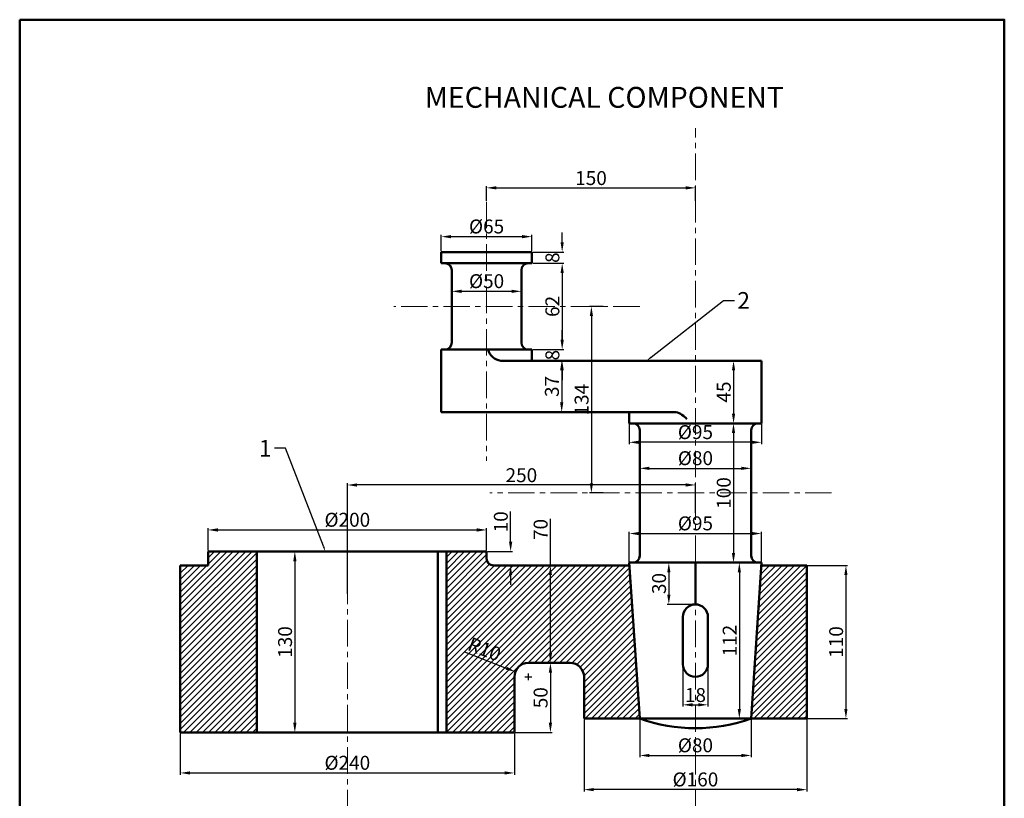
# Model space of a CAD drawing. Units: millimetres. Extents: x 1219 to 1926, y 574 to 1498.
# Tile 2 of 2: x 1219 to 1926, y 938 to 1498. Entities that reach past the tile are written whole.
import ezdxf
from ezdxf import colors
from ezdxf.entities.mleader import LeaderData, LeaderLine
from ezdxf.math import Vec2, Vec3

# ---------------------------------------------------------------- set-up
doc = ezdxf.new("R2010")
doc.units = ezdxf.units.MM
doc.header["$LTSCALE"] = 0.6
doc.linetypes.add('CENTER', pattern=[50.8, 31.75, -6.35, 6.35, -6.35])
for name, color, linetype, lineweight in [('M-CNTR', 1, 'CENTER', 18), ('M-DIMS', 2, 'Continuous', 25), ('M-HATC', 8, 'Continuous', 18), ('M-OUTL', 7, 'Continuous', 50), ('M-TEXT', 3, 'Continuous', 25), ('M-TTLB', 7, 'Continuous', 50)]:
    doc.layers.add(name, color=color, linetype=linetype, lineweight=lineweight)
doc.styles.get("Standard").update_dxf_attribs({"font": 'arial.ttf'})
doc.dimstyles.new('ISO-25', dxfattribs={"dimtxt": 10, "dimasz": 7, "dimexe": 1.25, "dimexo": 0.625, "dimtad": 1, "dimdec": 0, "dimtxsty": 'Standard', "dimcen": 2.5, "dimadec": 0, "dimazin": 0, "dimtfac": 1, "dimtdec": 0, "dimtofl": 0, "dimtmove": 0, "dimatfit": 3, "dimfxl": 1, "dimarcsym": 0})

# ---------------------------------------------------------------- blocks, each defined once
blk = doc.blocks.new('*D1')
at = {"layer": 'Defpoints', "color": 0, "ltscale": 0.6, "transparency": 16777216}
for p in [(1586.44, 1341.72), (1521.44, 1330.65), (1586.44, 1330.65)]:
    blk.add_point(p, dxfattribs=at)
at = {"layer": 'M-DIMS', "color": 0, "lineweight": -2, "ltscale": 0.6, "transparency": 16777216}
for p, q in [((1521.44, 1331.27), (1521.44, 1342.97)), ((1528.44, 1341.72), (1579.44, 1341.72)), ((1586.44, 1331.27), (1586.44, 1342.97))]:
    blk.add_line(p, q, dxfattribs=at)
at = {"layer": 'M-DIMS', "color": 0, "ltscale": 0.6, "transparency": 16777216}
for points in [[(1528.44, 1342.88), (1528.44, 1340.55), (1521.44, 1341.72)], [(1579.44, 1342.88), (1579.44, 1340.55), (1586.44, 1341.72)]]:
    blk.add_solid(points, dxfattribs=at)
at = {"layer": 'M-DIMS', "color": 0, "ltscale": 0.6, "transparency": 16777216, "insert": (1553.94, 1347.73), "char_height": 10, "attachment_point": 5}
blk.add_mtext('%%C65', dxfattribs=at)
blk = doc.blocks.new('*D2')
at = {"layer": 'Defpoints', "color": 0, "ltscale": 0.6, "transparency": 16777216}
for p in [(1703.94, 1376.76), (1553.94, 1366.8), (1703.94, 1366.8)]:
    blk.add_point(p, dxfattribs=at)
at = {"layer": 'M-DIMS', "color": 0, "lineweight": -2, "ltscale": 0.6, "transparency": 16777216}
for p, q in [((1553.94, 1367.43), (1553.94, 1378.01)), ((1560.94, 1376.76), (1696.94, 1376.76)), ((1703.94, 1367.43), (1703.94, 1378.01))]:
    blk.add_line(p, q, dxfattribs=at)
at = {"layer": 'M-DIMS', "color": 0, "ltscale": 0.6, "transparency": 16777216}
for points in [[(1560.94, 1377.93), (1560.94, 1375.6), (1553.94, 1376.76)], [(1696.94, 1377.93), (1696.94, 1375.6), (1703.94, 1376.76)]]:
    blk.add_solid(points, dxfattribs=at)
at = {"layer": 'M-DIMS', "color": 0, "ltscale": 0.6, "transparency": 16777216, "insert": (1628.94, 1382.49), "char_height": 10, "attachment_point": 5}
blk.add_mtext('150', dxfattribs=at)
blk = doc.blocks.new('*D3')
at = {"layer": 'Defpoints', "color": 0, "ltscale": 0.6, "transparency": 16777216}
for p in [(1586.44, 1330.65), (1586.44, 1322.65), (1608.23, 1322.65)]:
    blk.add_point(p, dxfattribs=at)
at = {"layer": 'M-DIMS', "color": 0, "lineweight": -2, "ltscale": 0.6, "transparency": 16777216}
for p, q in [((1608.23, 1337.65), (1608.23, 1344.65)), ((1587.07, 1330.65), (1609.48, 1330.65)), ((1587.07, 1322.65), (1609.48, 1322.65)), ((1608.23, 1315.65), (1608.23, 1308.65))]:
    blk.add_line(p, q, dxfattribs=at)
at = {"layer": 'M-DIMS', "color": 0, "ltscale": 0.6, "transparency": 16777216}
for points in [[(1607.06, 1337.65), (1609.4, 1337.65), (1608.23, 1330.65)], [(1607.06, 1315.65), (1609.4, 1315.65), (1608.23, 1322.65)]]:
    blk.add_solid(points, dxfattribs=at)
at = {"layer": 'M-DIMS', "color": 0, "ltscale": 0.6, "transparency": 16777216, "insert": (1602.5, 1326.65), "char_height": 10, "attachment_point": 5, "rotation": 90}
blk.add_mtext('8', dxfattribs=at)
blk = doc.blocks.new('*D4')
at = {"layer": 'Defpoints', "color": 0, "ltscale": 0.6, "transparency": 16777216}
for p in [(1586.44, 1322.65), (1586.44, 1260.65), (1608.23, 1260.65)]:
    blk.add_point(p, dxfattribs=at)
at = {"layer": 'M-DIMS', "color": 0, "lineweight": -2, "ltscale": 0.6, "transparency": 16777216}
for p, q in [((1587.07, 1322.65), (1609.48, 1322.65)), ((1608.23, 1315.65), (1608.23, 1267.65)), ((1587.07, 1260.65), (1609.48, 1260.65))]:
    blk.add_line(p, q, dxfattribs=at)
at = {"layer": 'M-DIMS', "color": 0, "ltscale": 0.6, "transparency": 16777216}
for points in [[(1607.06, 1315.65), (1609.4, 1315.65), (1608.23, 1322.65)], [(1607.06, 1267.65), (1609.4, 1267.65), (1608.23, 1260.65)]]:
    blk.add_solid(points, dxfattribs=at)
at = {"layer": 'M-DIMS', "color": 0, "ltscale": 0.6, "transparency": 16777216, "insert": (1602.5, 1291.65), "char_height": 10, "attachment_point": 5, "rotation": 90}
blk.add_mtext('62', dxfattribs=at)
blk = doc.blocks.new('*D5')
at = {"layer": 'Defpoints', "color": 0, "ltscale": 0.6, "transparency": 16777216}
for p in [(1586.44, 1260.65), (1586.44, 1252.65), (1608.23, 1252.65)]:
    blk.add_point(p, dxfattribs=at)
at = {"layer": 'M-DIMS', "color": 0, "lineweight": -2, "ltscale": 0.6, "transparency": 16777216}
for p, q in [((1608.23, 1267.65), (1608.23, 1274.65)), ((1587.07, 1260.65), (1609.48, 1260.65)), ((1587.07, 1252.65), (1609.48, 1252.65)), ((1608.23, 1245.65), (1608.23, 1238.65))]:
    blk.add_line(p, q, dxfattribs=at)
at = {"layer": 'M-DIMS', "color": 0, "ltscale": 0.6, "transparency": 16777216}
for points in [[(1607.06, 1267.65), (1609.4, 1267.65), (1608.23, 1260.65)], [(1607.06, 1245.65), (1609.4, 1245.65), (1608.23, 1252.65)]]:
    blk.add_solid(points, dxfattribs=at)
at = {"layer": 'M-DIMS', "color": 0, "ltscale": 0.6, "transparency": 16777216, "insert": (1602.5, 1256.65), "char_height": 10, "attachment_point": 5, "rotation": 90}
blk.add_mtext('8', dxfattribs=at)
blk = doc.blocks.new('*D6')
at = {"layer": 'Defpoints', "color": 0, "ltscale": 0.6, "transparency": 16777216}
for p in [(1616.05, 1252.65), (1607.9, 1215.65), (1616.05, 1215.65)]:
    blk.add_point(p, dxfattribs=at)
at = {"layer": 'M-DIMS', "color": 0, "lineweight": -2, "ltscale": 0.6, "transparency": 16777216}
for p, q in [((1615.42, 1252.65), (1606.65, 1252.65)), ((1607.9, 1245.65), (1607.9, 1222.65)), ((1615.42, 1215.65), (1606.65, 1215.65))]:
    blk.add_line(p, q, dxfattribs=at)
at = {"layer": 'M-DIMS', "color": 0, "ltscale": 0.6, "transparency": 16777216}
for points in [[(1606.73, 1245.65), (1609.06, 1245.65), (1607.9, 1252.65)], [(1606.73, 1222.65), (1609.06, 1222.65), (1607.9, 1215.65)]]:
    blk.add_solid(points, dxfattribs=at)
at = {"layer": 'M-DIMS', "color": 0, "ltscale": 0.6, "transparency": 16777216, "insert": (1602.16, 1234.15), "char_height": 10, "attachment_point": 5, "rotation": 90}
blk.add_mtext('37', dxfattribs=at)
blk = doc.blocks.new('*D7')
at = {"layer": 'Defpoints', "color": 0, "ltscale": 0.6, "transparency": 16777216}
for p in [(1638.23, 1291.65), (1629.22, 1157.65), (1638.23, 1157.65)]:
    blk.add_point(p, dxfattribs=at)
at = {"layer": 'M-DIMS', "color": 0, "lineweight": -2, "ltscale": 0.6, "transparency": 16777216}
for p, q in [((1637.61, 1291.65), (1627.97, 1291.65)), ((1629.22, 1284.65), (1629.22, 1164.65)), ((1637.61, 1157.65), (1627.97, 1157.65))]:
    blk.add_line(p, q, dxfattribs=at)
at = {"layer": 'M-DIMS', "color": 0, "ltscale": 0.6, "transparency": 16777216}
for points in [[(1628.06, 1284.65), (1630.39, 1284.65), (1629.22, 1291.65)], [(1628.06, 1164.65), (1630.39, 1164.65), (1629.22, 1157.65)]]:
    blk.add_solid(points, dxfattribs=at)
at = {"layer": 'M-DIMS', "color": 0, "ltscale": 0.6, "transparency": 16777216, "insert": (1623.49, 1224.65), "char_height": 10, "attachment_point": 5, "rotation": 90}
blk.add_mtext('134', dxfattribs=at)
blk = doc.blocks.new('*D8')
at = {"layer": 'Defpoints', "color": 0, "ltscale": 0.6, "transparency": 16777216}
for p in [(1528.94, 1303.11), (1578.94, 1303.11), (1578.94, 1302.46)]:
    blk.add_point(p, dxfattribs=at)
at = {"layer": 'M-DIMS', "color": 0, "lineweight": -2, "ltscale": 0.6, "transparency": 16777216}
for p, q in [((1528.94, 1302.48), (1528.94, 1301.21)), ((1535.94, 1302.46), (1571.94, 1302.46)), ((1578.94, 1302.48), (1578.94, 1301.21))]:
    blk.add_line(p, q, dxfattribs=at)
at = {"layer": 'M-DIMS', "color": 0, "ltscale": 0.6, "transparency": 16777216}
for points in [[(1535.94, 1303.63), (1535.94, 1301.29), (1528.94, 1302.46)], [(1571.94, 1303.63), (1571.94, 1301.29), (1578.94, 1302.46)]]:
    blk.add_solid(points, dxfattribs=at)
at = {"layer": 'M-DIMS', "color": 0, "ltscale": 0.6, "transparency": 16777216, "insert": (1553.94, 1308.47), "char_height": 10, "attachment_point": 5}
blk.add_mtext('%%C50', dxfattribs=at)
blk = doc.blocks.new('*D9')
at = {"layer": 'Defpoints', "color": 0, "ltscale": 0.6, "transparency": 16777216}
for p in [(1728.88, 1252.65), (1728.88, 1207.65), (1731.3, 1207.65)]:
    blk.add_point(p, dxfattribs=at)
at = {"layer": 'M-DIMS', "color": 0, "lineweight": -2, "ltscale": 0.6, "transparency": 16777216}
for p, q in [((1729.5, 1252.65), (1732.55, 1252.65)), ((1731.3, 1245.65), (1731.3, 1214.65)), ((1729.5, 1207.65), (1732.55, 1207.65))]:
    blk.add_line(p, q, dxfattribs=at)
at = {"layer": 'M-DIMS', "color": 0, "ltscale": 0.6, "transparency": 16777216}
for points in [[(1730.14, 1245.65), (1732.47, 1245.65), (1731.3, 1252.65)], [(1730.14, 1214.65), (1732.47, 1214.65), (1731.3, 1207.65)]]:
    blk.add_solid(points, dxfattribs=at)
at = {"layer": 'M-DIMS', "color": 0, "ltscale": 0.6, "transparency": 16777216, "insert": (1725.59, 1230.15), "char_height": 10, "attachment_point": 5, "rotation": 90}
blk.add_mtext('45', dxfattribs=at)
blk = doc.blocks.new('*D10')
at = {"layer": 'Defpoints', "color": 0, "ltscale": 0.6, "transparency": 16777216}
for p in [(1656.44, 1207.65), (1751.44, 1207.65), (1656.44, 1194.05)]:
    blk.add_point(p, dxfattribs=at)
at = {"layer": 'M-DIMS', "color": 0, "lineweight": -2, "ltscale": 0.6, "transparency": 16777216}
for p, q in [((1656.44, 1207.02), (1656.44, 1192.8)), ((1751.44, 1207.02), (1751.44, 1192.8)), ((1744.44, 1194.05), (1663.44, 1194.05))]:
    blk.add_line(p, q, dxfattribs=at)
at = {"layer": 'M-DIMS', "color": 0, "ltscale": 0.6, "transparency": 16777216}
for points in [[(1663.44, 1195.22), (1663.44, 1192.88), (1656.44, 1194.05)], [(1744.44, 1195.22), (1744.44, 1192.88), (1751.44, 1194.05)]]:
    blk.add_solid(points, dxfattribs=at)
at = {"layer": 'M-DIMS', "color": 0, "ltscale": 0.6, "transparency": 16777216, "insert": (1703.94, 1200.06), "char_height": 10, "attachment_point": 5}
blk.add_mtext('%%C95', dxfattribs=at)
blk = doc.blocks.new('*D11')
at = {"layer": 'Defpoints', "color": 0, "ltscale": 0.6, "transparency": 16777216}
for p in [(1663.94, 1175.97), (1743.94, 1175.97), (1743.94, 1175.35)]:
    blk.add_point(p, dxfattribs=at)
at = {"layer": 'M-DIMS', "color": 0, "lineweight": -2, "ltscale": 0.6, "transparency": 16777216}
for p, q in [((1663.94, 1175.35), (1663.94, 1174.1)), ((1670.94, 1175.35), (1736.94, 1175.35)), ((1743.94, 1175.35), (1743.94, 1174.1))]:
    blk.add_line(p, q, dxfattribs=at)
at = {"layer": 'M-DIMS', "color": 0, "ltscale": 0.6, "transparency": 16777216}
for points in [[(1670.94, 1176.52), (1670.94, 1174.19), (1663.94, 1175.35)], [(1736.94, 1176.52), (1736.94, 1174.19), (1743.94, 1175.35)]]:
    blk.add_solid(points, dxfattribs=at)
at = {"layer": 'M-DIMS', "color": 0, "ltscale": 0.6, "transparency": 16777216, "insert": (1703.94, 1181.36), "char_height": 10, "attachment_point": 5}
blk.add_mtext('%%C80', dxfattribs=at)
blk = doc.blocks.new('*D12')
at = {"layer": 'Defpoints', "color": 0, "ltscale": 0.6, "transparency": 16777216}
for p in [(1731.03, 1207.65), (1731.03, 1107.65), (1731.29, 1107.65)]:
    blk.add_point(p, dxfattribs=at)
at = {"layer": 'M-DIMS', "color": 0, "lineweight": -2, "ltscale": 0.6, "transparency": 16777216}
for p, q in [((1731.65, 1207.65), (1732.54, 1207.65)), ((1731.29, 1200.65), (1731.29, 1114.65)), ((1731.65, 1107.65), (1732.54, 1107.65))]:
    blk.add_line(p, q, dxfattribs=at)
at = {"layer": 'M-DIMS', "color": 0, "ltscale": 0.6, "transparency": 16777216}
for points in [[(1730.12, 1200.65), (1732.46, 1200.65), (1731.29, 1207.65)], [(1730.12, 1114.65), (1732.46, 1114.65), (1731.29, 1107.65)]]:
    blk.add_solid(points, dxfattribs=at)
at = {"layer": 'M-DIMS', "color": 0, "ltscale": 0.6, "transparency": 16777216, "insert": (1725.56, 1157.65), "char_height": 10, "attachment_point": 5, "rotation": 90}
blk.add_mtext('100', dxfattribs=at)
blk = doc.blocks.new('*D13')
at = {"layer": 'Defpoints', "color": 0, "ltscale": 0.6, "transparency": 16777216}
for p in [(1751.44, 1128.54), (1656.44, 1107.65), (1751.44, 1107.65)]:
    blk.add_point(p, dxfattribs=at)
at = {"layer": 'M-DIMS', "color": 0, "lineweight": -2, "ltscale": 0.6, "transparency": 16777216}
for p, q in [((1656.44, 1108.27), (1656.44, 1129.79)), ((1663.44, 1128.54), (1744.44, 1128.54)), ((1751.44, 1108.27), (1751.44, 1129.79))]:
    blk.add_line(p, q, dxfattribs=at)
at = {"layer": 'M-DIMS', "color": 0, "ltscale": 0.6, "transparency": 16777216}
for points in [[(1663.44, 1129.7), (1663.44, 1127.37), (1656.44, 1128.54)], [(1744.44, 1129.7), (1744.44, 1127.37), (1751.44, 1128.54)]]:
    blk.add_solid(points, dxfattribs=at)
at = {"layer": 'M-DIMS', "color": 0, "ltscale": 0.6, "transparency": 16777216, "insert": (1703.94, 1134.55), "char_height": 10, "attachment_point": 5}
blk.add_mtext('%%C95', dxfattribs=at)
blk = doc.blocks.new('*D14')
at = {"layer": 'Defpoints', "color": 0, "ltscale": 0.6, "transparency": 16777216}
for p in [(1703.94, 1107.65), (1684.83, 1077.65), (1703.94, 1077.65)]:
    blk.add_point(p, dxfattribs=at)
at = {"layer": 'M-DIMS', "color": 0, "lineweight": -2, "ltscale": 0.6, "transparency": 16777216}
for p, q in [((1703.32, 1107.65), (1683.58, 1107.65)), ((1684.83, 1100.65), (1684.83, 1084.65)), ((1703.32, 1077.65), (1683.58, 1077.65))]:
    blk.add_line(p, q, dxfattribs=at)
at = {"layer": 'M-DIMS', "color": 0, "ltscale": 0.6, "transparency": 16777216}
for points in [[(1683.67, 1100.65), (1686, 1100.65), (1684.83, 1107.65)], [(1683.67, 1084.65), (1686, 1084.65), (1684.83, 1077.65)]]:
    blk.add_solid(points, dxfattribs=at)
at = {"layer": 'M-DIMS', "color": 0, "ltscale": 0.6, "transparency": 16777216, "insert": (1679.1, 1092.65), "char_height": 10, "attachment_point": 5, "rotation": 90}
blk.add_mtext('30', dxfattribs=at)
blk = doc.blocks.new('*D15')
at = {"layer": 'Defpoints', "color": 0, "ltscale": 0.6, "transparency": 16777216}
for p in [(1731.03, 1107.65), (1731.03, 995.65), (1735.48, 995.65)]:
    blk.add_point(p, dxfattribs=at)
at = {"layer": 'M-DIMS', "color": 0, "lineweight": -2, "ltscale": 0.6, "transparency": 16777216}
for p, q in [((1731.65, 1107.65), (1736.73, 1107.65)), ((1735.48, 1100.65), (1735.48, 1002.65)), ((1731.65, 995.65), (1736.73, 995.65))]:
    blk.add_line(p, q, dxfattribs=at)
at = {"layer": 'M-DIMS', "color": 0, "ltscale": 0.6, "transparency": 16777216}
for points in [[(1734.31, 1100.65), (1736.65, 1100.65), (1735.48, 1107.65)], [(1734.31, 1002.65), (1736.65, 1002.65), (1735.48, 995.65)]]:
    blk.add_solid(points, dxfattribs=at)
at = {"layer": 'M-DIMS', "color": 0, "ltscale": 0.6, "transparency": 16777216, "insert": (1729.83, 1051.65), "char_height": 10, "attachment_point": 5, "rotation": 90}
blk.add_mtext('112', dxfattribs=at)
blk = doc.blocks.new('*D16')
at = {"layer": 'Defpoints', "color": 0, "ltscale": 0.6, "transparency": 16777216}
for p in [(1694.94, 1043.46), (1712.94, 1043.46), (1712.94, 1005.56)]:
    blk.add_point(p, dxfattribs=at)
at = {"layer": 'M-DIMS', "color": 0, "lineweight": -2, "ltscale": 0.6, "transparency": 16777216}
for p, q in [((1694.94, 1042.83), (1694.94, 1004.31)), ((1712.94, 1042.83), (1712.94, 1004.31)), ((1701.94, 1005.56), (1705.94, 1005.56))]:
    blk.add_line(p, q, dxfattribs=at)
at = {"layer": 'M-DIMS', "color": 0, "ltscale": 0.6, "transparency": 16777216}
for points in [[(1701.94, 1006.72), (1701.94, 1004.39), (1694.94, 1005.56)], [(1705.94, 1006.72), (1705.94, 1004.39), (1712.94, 1005.56)]]:
    blk.add_solid(points, dxfattribs=at)
at = {"layer": 'M-DIMS', "color": 0, "ltscale": 0.6, "transparency": 16777216, "insert": (1703.94, 1011.29), "char_height": 10, "attachment_point": 5}
blk.add_mtext('18', dxfattribs=at)
blk = doc.blocks.new('*D17')
at = {"layer": 'Defpoints', "color": 0, "ltscale": 0.6, "transparency": 16777216}
for p in [(1767.63, 1105.65), (1767.63, 995.65), (1812.01, 995.65)]:
    blk.add_point(p, dxfattribs=at)
at = {"layer": 'M-DIMS', "color": 0, "lineweight": -2, "ltscale": 0.6, "transparency": 16777216}
for p, q in [((1768.25, 1105.65), (1813.26, 1105.65)), ((1812.01, 1098.65), (1812.01, 1002.65)), ((1768.25, 995.65), (1813.26, 995.65))]:
    blk.add_line(p, q, dxfattribs=at)
at = {"layer": 'M-DIMS', "color": 0, "ltscale": 0.6, "transparency": 16777216}
for points in [[(1810.84, 1098.65), (1813.18, 1098.65), (1812.01, 1105.65)], [(1810.84, 1002.65), (1813.18, 1002.65), (1812.01, 995.65)]]:
    blk.add_solid(points, dxfattribs=at)
at = {"layer": 'M-DIMS', "color": 0, "ltscale": 0.6, "transparency": 16777216, "insert": (1806.28, 1050.65), "char_height": 10, "attachment_point": 5, "rotation": 90}
blk.add_mtext('110', dxfattribs=at)
blk = doc.blocks.new('*D18')
at = {"layer": 'Defpoints', "color": 0, "ltscale": 0.6, "transparency": 16777216}
for p in [(1553.94, 1131.12), (1353.94, 1115.65), (1553.94, 1115.65)]:
    blk.add_point(p, dxfattribs=at)
at = {"layer": 'M-DIMS', "color": 0, "lineweight": -2, "ltscale": 0.6, "transparency": 16777216}
for p, q in [((1353.94, 1116.27), (1353.94, 1132.37)), ((1553.94, 1116.27), (1553.94, 1132.37)), ((1360.94, 1131.12), (1546.94, 1131.12))]:
    blk.add_line(p, q, dxfattribs=at)
at = {"layer": 'M-DIMS', "color": 0, "ltscale": 0.6, "transparency": 16777216}
for points in [[(1360.94, 1132.29), (1360.94, 1129.95), (1353.94, 1131.12)], [(1546.94, 1132.29), (1546.94, 1129.95), (1553.94, 1131.12)]]:
    blk.add_solid(points, dxfattribs=at)
at = {"layer": 'M-DIMS', "color": 0, "ltscale": 0.6, "transparency": 16777216, "insert": (1453.94, 1137.13), "char_height": 10, "attachment_point": 5}
blk.add_mtext('%%C200', dxfattribs=at)
blk = doc.blocks.new('*D19')
at = {"layer": 'Defpoints', "color": 0, "ltscale": 0.6, "transparency": 16777216}
for p in [(1453.94, 1163.41), (1703.94, 1142.52), (1453.94, 1084.55)]:
    blk.add_point(p, dxfattribs=at)
at = {"layer": 'M-DIMS', "color": 0, "lineweight": -2, "ltscale": 0.6, "transparency": 16777216}
for p, q in [((1453.94, 1085.17), (1453.94, 1164.66)), ((1696.94, 1163.41), (1460.94, 1163.41)), ((1703.94, 1143.14), (1703.94, 1164.66))]:
    blk.add_line(p, q, dxfattribs=at)
at = {"layer": 'M-DIMS', "color": 0, "ltscale": 0.6, "transparency": 16777216}
for points in [[(1460.94, 1164.57), (1460.94, 1162.24), (1453.94, 1163.41)], [(1696.94, 1164.57), (1696.94, 1162.24), (1703.94, 1163.41)]]:
    blk.add_solid(points, dxfattribs=at)
at = {"layer": 'M-DIMS', "color": 0, "ltscale": 0.6, "transparency": 16777216, "insert": (1578.94, 1169.14), "char_height": 10, "attachment_point": 5}
blk.add_mtext('250', dxfattribs=at)
blk = doc.blocks.new('*D20')
at = {"layer": 'Defpoints', "color": 0, "ltscale": 0.6, "transparency": 16777216}
for p in [(1333.94, 985.65), (1573.94, 985.65), (1573.94, 956.62)]:
    blk.add_point(p, dxfattribs=at)
at = {"layer": 'M-DIMS', "color": 0, "lineweight": -2, "ltscale": 0.6, "transparency": 16777216}
for p, q in [((1333.94, 985.02), (1333.94, 955.37)), ((1573.94, 985.02), (1573.94, 955.37)), ((1340.94, 956.62), (1566.94, 956.62))]:
    blk.add_line(p, q, dxfattribs=at)
at = {"layer": 'M-DIMS', "color": 0, "ltscale": 0.6, "transparency": 16777216}
for points in [[(1340.94, 957.79), (1340.94, 955.46), (1333.94, 956.62)], [(1566.94, 957.79), (1566.94, 955.46), (1573.94, 956.62)]]:
    blk.add_solid(points, dxfattribs=at)
at = {"layer": 'M-DIMS', "color": 0, "ltscale": 0.6, "transparency": 16777216, "insert": (1453.94, 962.63), "char_height": 10, "attachment_point": 5}
blk.add_mtext('%%C240', dxfattribs=at)
blk = doc.blocks.new('*D21')
at = {"layer": 'Defpoints', "color": 0, "ltscale": 0.6, "transparency": 16777216}
for p in [(1416.57, 1115.65), (1416.23, 985.65), (1416.57, 985.65)]:
    blk.add_point(p, dxfattribs=at)
at = {"layer": 'M-DIMS', "color": 0, "lineweight": -2, "ltscale": 0.6, "transparency": 16777216}
for p, q in [((1415.94, 1115.65), (1414.98, 1115.65)), ((1416.23, 1108.65), (1416.23, 992.65)), ((1415.94, 985.65), (1414.98, 985.65))]:
    blk.add_line(p, q, dxfattribs=at)
at = {"layer": 'M-DIMS', "color": 0, "ltscale": 0.6, "transparency": 16777216}
for points in [[(1415.07, 1108.65), (1417.4, 1108.65), (1416.23, 1115.65)], [(1415.07, 992.65), (1417.4, 992.65), (1416.23, 985.65)]]:
    blk.add_solid(points, dxfattribs=at)
at = {"layer": 'M-DIMS', "color": 0, "ltscale": 0.6, "transparency": 16777216, "insert": (1410.5, 1050.65), "char_height": 10, "attachment_point": 5, "rotation": 90}
blk.add_mtext('130', dxfattribs=at)
blk = doc.blocks.new('*D22')
at = {"layer": 'Defpoints', "color": 0, "ltscale": 0.6, "transparency": 16777216}
for p in [(1623.94, 995.65), (1783.94, 995.65), (1623.94, 944.65)]:
    blk.add_point(p, dxfattribs=at)
at = {"layer": 'M-DIMS', "color": 0, "lineweight": -2, "ltscale": 0.6, "transparency": 16777216}
for p, q in [((1623.94, 995.02), (1623.94, 943.4)), ((1783.94, 995.02), (1783.94, 943.4)), ((1776.94, 944.65), (1630.94, 944.65))]:
    blk.add_line(p, q, dxfattribs=at)
at = {"layer": 'M-DIMS', "color": 0, "ltscale": 0.6, "transparency": 16777216}
for points in [[(1630.94, 945.82), (1630.94, 943.48), (1623.94, 944.65)], [(1776.94, 945.82), (1776.94, 943.48), (1783.94, 944.65)]]:
    blk.add_solid(points, dxfattribs=at)
at = {"layer": 'M-DIMS', "color": 0, "ltscale": 0.6, "transparency": 16777216, "insert": (1703.94, 950.66), "char_height": 10, "attachment_point": 5}
blk.add_mtext('%%C160', dxfattribs=at)
blk = doc.blocks.new('*D23')
at = {"layer": 'Defpoints', "color": 0, "ltscale": 0.6, "transparency": 16777216}
for p in [(1663.94, 995.65), (1743.94, 995.65), (1743.94, 969.17)]:
    blk.add_point(p, dxfattribs=at)
at = {"layer": 'M-DIMS', "color": 0, "lineweight": -2, "ltscale": 0.6, "transparency": 16777216}
for p, q in [((1663.94, 995.02), (1663.94, 967.92)), ((1743.94, 995.02), (1743.94, 967.92)), ((1670.94, 969.17), (1736.94, 969.17))]:
    blk.add_line(p, q, dxfattribs=at)
at = {"layer": 'M-DIMS', "color": 0, "ltscale": 0.6, "transparency": 16777216}
for points in [[(1670.94, 970.34), (1670.94, 968.01), (1663.94, 969.17)], [(1736.94, 970.34), (1736.94, 968.01), (1743.94, 969.17)]]:
    blk.add_solid(points, dxfattribs=at)
at = {"layer": 'M-DIMS', "color": 0, "ltscale": 0.6, "transparency": 16777216, "insert": (1703.94, 975.18), "char_height": 10, "attachment_point": 5}
blk.add_mtext('%%C80', dxfattribs=at)
blk = doc.blocks.new('*D24')
at = {"layer": 'Defpoints', "color": 0, "ltscale": 0.6, "transparency": 16777216}
for p in [(1553.94, 1115.65), (1571.21, 1105.65), (1572.84, 1105.65)]:
    blk.add_point(p, dxfattribs=at)
at = {"layer": 'M-DIMS', "color": 0, "lineweight": -2, "ltscale": 0.6, "transparency": 16777216}
for p, q in [((1571.21, 1122.65), (1571.21, 1144.25)), ((1554.57, 1115.65), (1572.46, 1115.65)), ((1572.21, 1105.65), (1569.96, 1105.65)), ((1571.21, 1098.65), (1571.21, 1091.65))]:
    blk.add_line(p, q, dxfattribs=at)
at = {"layer": 'M-DIMS', "color": 0, "ltscale": 0.6, "transparency": 16777216}
for points in [[(1570.04, 1122.65), (1572.37, 1122.65), (1571.21, 1115.65)], [(1570.04, 1098.65), (1572.37, 1098.65), (1571.21, 1105.65)]]:
    blk.add_solid(points, dxfattribs=at)
at = {"layer": 'M-DIMS', "color": 0, "ltscale": 0.6, "transparency": 16777216, "insert": (1565.48, 1136.95), "char_height": 10, "attachment_point": 5, "rotation": 90}
blk.add_mtext('10', dxfattribs=at)
blk = doc.blocks.new('*D25')
at = {"layer": 'Defpoints', "color": 0, "ltscale": 0.6, "transparency": 16777216}
for p in [(1599.79, 1105.65), (1599.79, 1035.65), (1599.79, 1035.65)]:
    blk.add_point(p, dxfattribs=at)
at = {"layer": 'M-DIMS', "color": 0, "lineweight": -2, "ltscale": 0.6, "transparency": 16777216}
for p, q in [((1599.79, 1105.65), (1599.79, 1139.18)), ((1599.16, 1105.65), (1598.54, 1105.65)), ((1599.79, 1042.65), (1599.79, 1098.65)), ((1599.16, 1035.65), (1598.54, 1035.65))]:
    blk.add_line(p, q, dxfattribs=at)
at = {"layer": 'M-DIMS', "color": 0, "ltscale": 0.6, "transparency": 16777216}
for points in [[(1598.62, 1098.65), (1600.95, 1098.65), (1599.79, 1105.65)], [(1598.62, 1042.65), (1600.95, 1042.65), (1599.79, 1035.65)]]:
    blk.add_solid(points, dxfattribs=at)
at = {"layer": 'M-DIMS', "color": 0, "ltscale": 0.6, "transparency": 16777216, "insert": (1594.06, 1131.45), "char_height": 10, "attachment_point": 5, "rotation": 90}
blk.add_mtext('70', dxfattribs=at)
blk = doc.blocks.new('*D26')
at = {"layer": 'Defpoints', "color": 0, "ltscale": 0.6, "transparency": 16777216}
for p in [(1595.89, 1035.65), (1573.94, 985.65), (1599.79, 985.65)]:
    blk.add_point(p, dxfattribs=at)
at = {"layer": 'M-DIMS', "color": 0, "lineweight": -2, "ltscale": 0.6, "transparency": 16777216}
for p, q in [((1596.52, 1035.65), (1601.04, 1035.65)), ((1599.79, 1028.65), (1599.79, 992.65)), ((1574.57, 985.65), (1601.04, 985.65))]:
    blk.add_line(p, q, dxfattribs=at)
at = {"layer": 'M-DIMS', "color": 0, "ltscale": 0.6, "transparency": 16777216}
for points in [[(1598.62, 1028.65), (1600.95, 1028.65), (1599.79, 1035.65)], [(1598.62, 992.65), (1600.95, 992.65), (1599.79, 985.65)]]:
    blk.add_solid(points, dxfattribs=at)
at = {"layer": 'M-DIMS', "color": 0, "ltscale": 0.6, "transparency": 16777216, "insert": (1594.06, 1010.65), "char_height": 10, "attachment_point": 5, "rotation": 90}
blk.add_mtext('50', dxfattribs=at)
blk = doc.blocks.new('*D27')
at = {"layer": 'Defpoints', "color": 0, "ltscale": 0.6, "transparency": 16777216}
for p in [(1574.63, 1029.29), (1583.94, 1025.65)]:
    blk.add_point(p, dxfattribs=at)
at = {"layer": 'M-DIMS', "color": 0, "lineweight": -2, "ltscale": 0.6, "transparency": 16777216}
for p, q in [((1538.2, 1043.52), (1568.11, 1031.84)), ((1581.44, 1025.65), (1586.44, 1025.65)), ((1583.94, 1023.15), (1583.94, 1028.15))]:
    blk.add_line(p, q, dxfattribs=at)
at = {"layer": 'M-DIMS', "color": 0, "ltscale": 0.6, "transparency": 16777216}
blk.add_solid([(1568.53, 1032.92), (1567.68, 1030.75), (1574.63, 1029.29)], dxfattribs=at)
at = {"layer": 'M-DIMS', "color": 0, "ltscale": 0.6, "transparency": 16777216, "insert": (1551.98, 1044.29), "char_height": 10, "attachment_point": 5, "rotation": 338.65957}
blk.add_mtext('R10', dxfattribs=at)

msp = doc.modelspace()

# ---------------------------------------------------------------- hatches: boundary and pattern name
at = {"layer": 'M-HATC', "ltscale": 0.6}
h = msp.add_hatch(dxfattribs=at)
h.set_pattern_fill('ANSI31', color=256)
h.set_pattern_definition([(45, (1329.0515, 767.3282), (-2.245064, 2.245064), [])])
h.paths.add_polyline_path([(1525.11, 985.65), (1573.94, 985.65), (1573.94, 1025.65, -0.414214), (1583.94, 1035.65), (1613.94, 1035.65, -0.414214), (1623.94, 1025.65), (1623.94, 995.65), (1663.94, 995.65), (1656.58, 1105.65), (1558.94, 1105.65, -0.414214), (1553.94, 1110.65), (1553.94, 1115.65), (1525.11, 1115.65)])
h.paths.add_polyline_path([(1388.94, 1115.65), (1353.94, 1115.65), (1353.94, 1105.65), (1333.94, 1105.65), (1333.94, 995.65), (1333.94, 985.65), (1388.94, 985.65)])
h.paths.add_polyline_path([(1783.94, 1105.65), (1751.31, 1105.65), (1743.94, 995.65), (1783.94, 995.65)])

# ---------------------------------------------------------------- linework, layer by layer
at = {"layer": 'M-CNTR'}
for p, q in [((1703.94, 620.33), (1703.94, 1419.58)), ((1553.94, 1366.8), (1553.94, 1180.82)), ((1663.94, 1291.65), (1487.31, 1291.65)), ((1801.77, 1157.65), (1556.33, 1157.65)), ((1453.94, 620.73), (1453.94, 1146.58))]:
    msp.add_line(p, q, dxfattribs=at)
at = {"layer": 'M-OUTL'}
for p, q in [((1521.44, 1330.65), (1586.44, 1330.65)), ((1521.44, 1322.65), (1521.44, 1330.65)), ((1586.44, 1330.65), (1586.44, 1322.65)), ((1523.94, 1322.65), (1521.44, 1322.65)), ((1586.44, 1322.65), (1523.94, 1322.65)), ((1528.94, 1317.65), (1528.94, 1265.65)), ((1578.94, 1317.65), (1578.94, 1265.65)), ((1521.44, 1252.65), (1521.44, 1260.65)), ((1521.44, 1260.65), (1523.94, 1260.65)), ((1523.94, 1260.65), (1586.44, 1260.65)), ((1586.44, 1260.65), (1586.44, 1252.65)), ((1521.44, 1252.65), (1521.44, 1215.65)), ((1586.44, 1252.65), (1564.15, 1252.65)), ((1751.44, 1252.65), (1586.44, 1252.65)), ((1751.44, 1207.65), (1751.44, 1252.65)), ((1521.44, 1215.65), (1689.85, 1215.65)), ((1656.44, 1207.65), (1656.44, 1215.65)), ((1748.94, 1207.65), (1656.44, 1207.65)), ((1663.94, 1112.65), (1663.94, 1202.65)), ((1743.94, 1112.65), (1743.94, 1202.65)), ((1751.44, 1207.65), (1748.94, 1207.65)), ((1353.94, 1105.65), (1353.94, 1115.65)), ((1553.94, 1115.65), (1353.94, 1115.65)), ((1553.94, 1110.65), (1553.94, 1115.65)), ((1333.94, 995.65), (1333.94, 1105.65)), ((1353.94, 1105.65), (1333.94, 1105.65)), ((1656.58, 1105.65), (1558.94, 1105.65)), ((1656.44, 1107.65), (1663.94, 995.65)), ((1658.94, 1107.65), (1656.44, 1107.65)), ((1751.44, 1107.65), (1658.94, 1107.65)), ((1751.44, 1107.65), (1743.94, 995.65)), ((1783.94, 1105.65), (1751.31, 1105.65)), ((1783.94, 995.65), (1783.94, 1105.65)), ((1583.94, 1035.65), (1613.94, 1035.65)), ((1573.94, 985.65), (1573.94, 1025.65)), ((1623.94, 995.65), (1623.94, 1025.65)), ((1333.94, 995.65), (1333.94, 985.65)), ((1623.94, 995.65), (1783.94, 995.65)), ((1663.94, 995.65), (1743.94, 995.65)), ((1333.94, 985.65), (1573.94, 985.65))]:
    msp.add_line(p, q, dxfattribs=at)
at = {"layer": 'M-OUTL', "ltscale": 0.6}
for p, q in [((1388.94, 985.65), (1388.94, 1115.65)), ((1518.94, 985.65), (1518.94, 1115.65)), ((1525.11, 985.65), (1525.11, 1115.65)), ((1703.94, 1107.65), (1703.94, 1077.65)), ((1694.94, 1034.65), (1694.94, 1068.65)), ((1712.94, 1068.65), (1712.94, 1034.65))]:
    msp.add_line(p, q, dxfattribs=at)
at = {"layer": 'M-OUTL'}
for centre, radius, start, end in [((1523.94, 1317.65), 5, 0, 90), ((1583.94, 1317.65), 5, 90, 180), ((1523.94, 1265.65), 5, 270, 0), ((1583.94, 1265.65), 5, 180, 270), ((1686.95, 1202.28), 13.68, 37.48485, 77.77972), ((1658.94, 1202.65), 5, 0, 90), ((1748.94, 1202.65), 5, 90, 180), ((1558.94, 1110.65), 5, 180, 270), ((1658.94, 1112.65), 5, 270, 0), ((1748.94, 1112.65), 5, 180, 270), ((1583.94, 1025.65), 10, 90, 180), ((1613.94, 1025.65), 10, 0, 90), ((1703.94, 1108.79), 120, 250.52878, 289.47122)]:
    msp.add_arc(centre, radius, start, end, dxfattribs=at)
at = {"layer": 'M-OUTL', "ltscale": 0.6}
for centre, radius, start, end in [((1565.15, 1262.78), 10.19, 192.10329, 264.33297), ((1703.94, 1068.65), 9, 0, 180), ((1703.94, 1034.65), 9, 180, 0)]:
    msp.add_arc(centre, radius, start, end, dxfattribs=at)
at = {"layer": 'M-TTLB', "ltscale": 0.6}
msp.add_lwpolyline([(1218.63, 1497.51), (1925.77, 1497.51), (1925.77, 573.72), (1218.63, 573.72)], close=True, dxfattribs=at)

# ---------------------------------------------------------------- texts
at = {"layer": 'M-TEXT', "ltscale": 0.6, "insert": (1489.11, 1449.24), "char_height": 15, "attachment_point": 1}
msp.add_mtext_dynamic_manual_height_columns('\\pxqc;MECHANICAL COMPONENT', width=298.8576, gutter_width=12.5, heights=[0], dxfattribs=at)

# ---------------------------------------------------------------- dimensions: what is measured, and where the dimension line sits
at = {"layer": 'M-DIMS', "ltscale": 0.6}
for base, p1, p2, picture, middle in [((1703.94, 1376.76), (1553.94, 1366.8), (1703.94, 1366.8), '*D2', (1628.94, 1382.49)), ((1453.94, 1163.41), (1703.94, 1142.52), (1453.94, 1084.55), '*D19', (1578.94, 1169.14)), ((1712.94, 1005.56), (1694.94, 1043.46), (1712.94, 1043.46), '*D16', (1703.94, 1011.29))]:
    dim = msp.add_linear_dim(base=base, p1=p1, p2=p2, dimstyle='ISO-25', override={"dimclrd": 0, "dimclre": 0, "dimclrt": 0}, dxfattribs=at)
    dim.commit()
    dim.dimension.update_dxf_attribs({"geometry": picture, "text_midpoint": middle})
for base, p1, p2, picture, middle in [((1586.44, 1341.72), (1521.44, 1330.65), (1586.44, 1330.65), '*D1', (1553.94, 1347.73)), ((1578.94, 1302.46), (1528.94, 1303.11), (1578.94, 1303.11), '*D8', (1553.94, 1308.47)), ((1656.44, 1194.05), (1751.44, 1207.65), (1656.44, 1207.65), '*D10', (1703.94, 1200.06)), ((1553.94, 1131.12), (1353.94, 1115.65), (1553.94, 1115.65), '*D18', (1453.94, 1137.13)), ((1573.94, 956.62), (1333.94, 985.65), (1573.94, 985.65), '*D20', (1453.94, 962.63))]:
    dim = msp.add_linear_dim(base=base, p1=p1, p2=p2, text='%%C<>', dimstyle='ISO-25', override={"dimclrd": 0, "dimclre": 0, "dimclrt": 0}, dxfattribs=at)
    dim.commit()
    dim.dimension.update_dxf_attribs({"geometry": picture, "text_midpoint": middle})
for base, p1, p2, picture, middle in [((1608.23, 1322.65), (1586.44, 1330.65), (1586.44, 1322.65), '*D3', (1602.5, 1326.65)), ((1608.23, 1260.65), (1586.44, 1322.65), (1586.44, 1260.65), '*D4', (1602.5, 1291.65)), ((1629.22, 1157.65), (1638.23, 1291.65), (1638.23, 1157.65), '*D7', (1623.49, 1224.65)), ((1608.23, 1252.65), (1586.44, 1260.65), (1586.44, 1252.65), '*D5', (1602.5, 1256.65)), ((1607.9, 1215.65), (1616.05, 1252.65), (1616.05, 1215.65), '*D6', (1602.16, 1234.15)), ((1731.3, 1207.65), (1728.88, 1252.65), (1728.88, 1207.65), '*D9', (1725.59, 1230.15)), ((1731.29, 1107.65), (1731.03, 1207.65), (1731.03, 1107.65), '*D12', (1725.56, 1157.65)), ((1416.23, 985.65), (1416.57, 1115.65), (1416.57, 985.65), '*D21', (1410.5, 1050.65)), ((1684.83, 1077.65), (1703.94, 1107.65), (1703.94, 1077.65), '*D14', (1679.1, 1092.65)), ((1735.48, 995.65), (1731.03, 1107.65), (1731.03, 995.65), '*D15', (1729.83, 1051.65)), ((1812.01, 995.65), (1767.63, 1105.65), (1767.63, 995.65), '*D17', (1806.28, 1050.65)), ((1599.79, 985.65), (1595.89, 1035.65), (1573.94, 985.65), '*D26', (1594.06, 1010.65))]:
    dim = msp.add_linear_dim(base=base, p1=p1, p2=p2, angle=90, dimstyle='ISO-25', override={"dimclrd": 0, "dimclre": 0, "dimclrt": 0}, dxfattribs=at)
    dim.commit()
    dim.dimension.update_dxf_attribs({"geometry": picture, "text_midpoint": middle})
for base, p1, p2, picture, middle in [((1743.94, 1175.35), (1663.94, 1175.97), (1743.94, 1175.97), '*D11', (1703.94, 1175.35)), ((1751.44, 1128.54), (1656.44, 1107.65), (1751.44, 1107.65), '*D13', (1703.94, 1128.54)), ((1623.94, 944.65), (1783.94, 995.65), (1623.94, 995.65), '*D22', (1703.94, 944.65)), ((1743.94, 969.17), (1663.94, 995.65), (1743.94, 995.65), '*D23', (1703.94, 969.17))]:
    dim = msp.add_linear_dim(base=base, p1=p1, p2=p2, text='%%C<>', dimstyle='ISO-25', override={"dimclrd": 0, "dimclre": 0, "dimclrt": 0}, dxfattribs=at)
    dim.commit()
    dim.dimension.update_dxf_attribs({"geometry": picture, "text_midpoint": middle, "dimtype": 160})
for base, p1, p2, picture, middle in [((1571.21, 1105.65), (1553.94, 1115.65), (1572.84, 1105.65), '*D24', (1571.21, 1136.95)), ((1599.79, 1035.65), (1599.79, 1105.65), (1599.79, 1035.65), '*D25', (1599.79, 1131.45))]:
    dim = msp.add_linear_dim(base=base, p1=p1, p2=p2, angle=90, dimstyle='ISO-25', override={"dimclrd": 0, "dimclre": 0, "dimclrt": 0}, dxfattribs=at)
    dim.commit()
    dim.dimension.update_dxf_attribs({"geometry": picture, "text_midpoint": middle, "dimtype": 160})
dim = msp.add_radius_dim(center=(1583.94, 1025.65), mpoint=(1574.63, 1029.29), dimstyle='ISO-25', override={"dimclrd": 0, "dimclre": 0, "dimclrt": 0}, dxfattribs=at)
dim.commit()
dim.dimension.update_dxf_attribs({"geometry": '*D27', "text_midpoint": (1551.98, 1044.29)})

# ---------------------------------------------------------------- leaders
at = {"layer": 'M-TEXT', "ltscale": 0.6}
ml = msp.add_multileader_mtext('Standard', dxfattribs=at)
ml.set_content('2', color=256)
ml.set_leader_properties()
ml.build(insert=Vec2(0, 0))
ctx = ml.context
ctx.base_point, ctx.char_height, ctx.plane_origin = Vec3(1732.02, 1295.91), 12, Vec3(1668.94, 1252.65)
notes = []
notes.append((ctx, [(0, (1, 1, 0), (1724.02, 1295.91), (1, 0), 8, [(0, [(1668.94, 1252.65)], 0, [])])]))
ctx.mtext.insert, ctx.mtext.flow_direction = Vec3(1734.02, 1301.91), 5
ml = msp.add_multileader_mtext('Standard', dxfattribs=at)
ml.set_content('1', color=256)
ml.set_leader_properties()
ml.build(insert=Vec2(0, 0))
ctx = ml.context
ctx.base_point, ctx.char_height, ctx.plane_origin = Vec3(1393.14, 1189.79), 12, Vec3(1438.2, 1115.65)
ctx.text_align_type = 2
notes.append((ctx, [(0, (1, 1, 0), (1409.56, 1189.79), (-1, 0), 8, [(0, [(1438.2, 1115.65)], 0, [])])]))
ctx.mtext.insert, ctx.mtext.alignment, ctx.mtext.flow_direction = Vec3(1399.56, 1195.79), 3, 5
for ctx, leaders in notes:
    for number, flags, end, landing, length, lines in leaders:
        leader = LeaderData()
        leader.index, (leader.has_last_leader_line, leader.has_dogleg_vector, leader.attachment_direction) = number, flags
        leader.last_leader_point, leader.dogleg_vector, leader.dogleg_length = Vec3(end), Vec3(landing), length
        for number, points, colour, breaks in lines:
            line = LeaderLine()
            line.index, line.vertices, line.color, line.breaks = number, Vec3.list(points), colors.encode_raw_color(colour), breaks
            leader.lines.append(line)
        ctx.leaders.append(leader)

doc.saveas('drawing.dxf')
